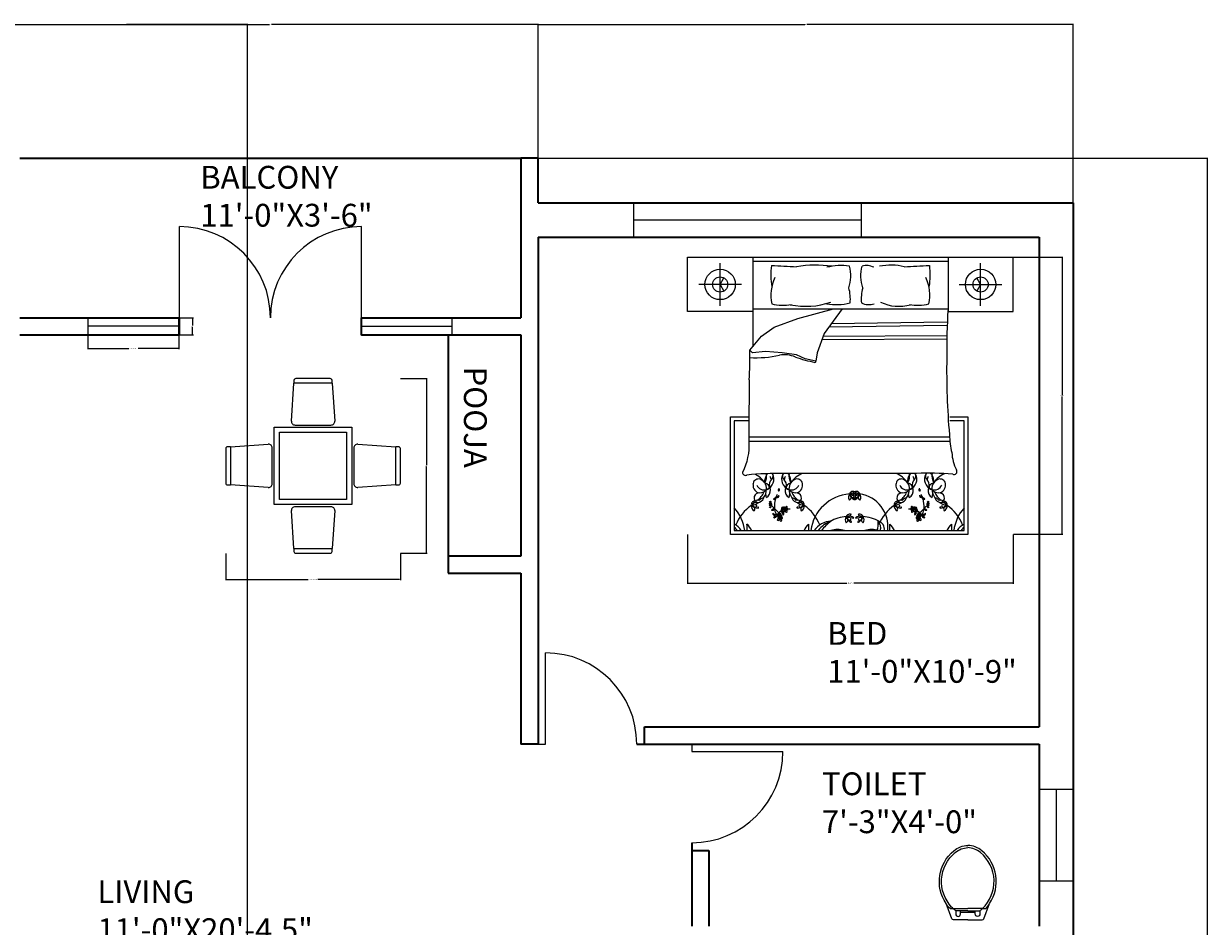
# Model space of a CAD drawing. Units: inches. Extents: x -59 to 444, y -680 to 63.
# Tile 9 of 9: x 132 to 444, y -175 to 63. Entities that reach past the tile are written whole.
import ezdxf

# ---------------------------------------------------------------- set-up
doc = ezdxf.new("R2010")
doc.units = ezdxf.units.IN
doc.header["$MEASUREMENT"] = 0
for name, color, linetype, lineweight in [('A-ANNO-DIMS', 2, 'Continuous', 18), ('A-AREA-IDEN', 7, 'Continuous', 18), ('A-DOOR', 3, 'Continuous', 18), ('A-FLOR-FIXT', 9, 'Continuous', 18), ('A-FURN', 8, 'Continuous', 13), ('A-GLAZ', 4, 'Continuous', 18), ('A-WALL', 7, 'Continuous', 35)]:
    doc.layers.add(name, color=color, linetype=linetype, lineweight=lineweight)
doc.styles.get("Standard").update_dxf_attribs({"font": 'arial.ttf'})
doc.dimstyles.get("Standard").update_dxf_attribs({"dimtxt": 0.18, "dimasz": 0.18, "dimexe": 0.18, "dimexo": 0.0625, "dimgap": 0.09, "dimtad": 0, "dimtih": 1, "dimtoh": 1, "dimdec": 0, "dimzin": 0, "dimdsep": 46, "dimlunit": 3, "dimtxsty": 'Standard', "dimcen": 0.09, "dimadec": 0, "dimazin": 0, "dimtfac": 1, "dimtdec": 0, "dimtofl": 0, "dimtmove": 0, "dimatfit": 3, "dimfxl": 1, "dimtolj": 1, "dimtzin": 0, "dimarcsym": 0})

# ---------------------------------------------------------------- blocks, each defined once
blk = doc.blocks.new('BED-SET-73')
for p, q in [((0, 72.95), (85.77, 72.95)), ((17.15, 72.95), (17.15, 49.4)), ((68.62, 71.84), (17.15, 71.84)), ((8.58, 60.19), (8.58, 71.4)), ((77.2, 60.19), (77.2, 71.4)), ((14.18, 65.8), (2.97, 65.8)), ((71.59, 65.8), (82.8, 65.8)), ((17.15, 59.39), (68.62, 59.39)), ((29.07, 56.84), (38.42, 59.39)), ((40.72, 59.39), (36.02, 52.85)), ((22.81, 54.58), (29.07, 56.84)), ((19.51, 52.15), (22.81, 54.58)), ((68.36, 54.95), (37.21, 54.51)), ((68.39, 55.83), (37.85, 55.4)), ((16.39, 48.51), (19.51, 52.15)), ((36.02, 52.85), (34.11, 47.81)), ((68.32, 51.37), (35.4, 51.23)), ((68.31, 52.25), (35.74, 52.12)), ((17.08, 47.81), (16.39, 48.51)), ((20.56, 48.16), (17.08, 47.81)), ((24.9, 47.81), (20.56, 48.16)), ((28.72, 47.29), (24.9, 47.81)), ((30.98, 46.25), (28.72, 47.29)), ((34.11, 47.81), (33.76, 45.56)), ((33.76, 45.56), (30.98, 46.25)), ((11.32, 30.9), (16.17, 30.9)), ((11.32, 0), (11.32, 30.9)), ((16.17, 29.9), (12.32, 29.9)), ((12.32, 29.9), (12.32, 0.99)), ((72.86, 29.9), (69.08, 29.9)), ((69.1, 30.9), (73.85, 30.9)), ((72.86, 0.99), (72.86, 29.9)), ((73.85, 30.9), (73.85, 0)), ((69.01, 25.55), (16.17, 25.55)), ((69.09, 24.48), (16.17, 24.48)), ((60.3, 16.05), (25.47, 16.05)), ((20.77, 9.69), (20.58, 10.66)), ((26.76, 9.69), (26.95, 10.66)), ((58.41, 9.69), (58.22, 10.66)), ((64.41, 9.69), (64.6, 10.66)), ((73.85, 0), (11.32, 0)), ((12.32, 0.99), (72.86, 0.99))]:
    blk.add_line(p, q)
for points in [[(17.15, 58.65), (0, 58.65), (0, 72.95)], [(68.62, 72.95), (68.62, 58.65), (85.77, 58.65), (85.77, 72.95)], [(8.58, 65.8), (9.58, 67.53)], [(8.58, 65.8), (9.58, 64.06)], [(77.2, 65.8), (76.2, 67.53)], [(77.2, 65.8), (76.2, 64.06)]]:
    blk.add_lwpolyline(points)
for points in [[(22.08, 70.81, 0.074897), (22.19, 65.21, -0.472817)], [(42.49, 64.89, 0.14099), (42.66, 70.61, 0.235245)], [(46.15, 64.89, -0.14099), (45.98, 70.61, -0.235245)], [(63.69, 70.81, -0.074897), (63.59, 65.21, 0.472817)], [(16.21, 40.65, 0.001242), (16.17, 24.38, -0.127202), (14.45, 16.27)], [(68.99, 26.22, 0.056112), (69.61, 21.51, 0.095341), (70.81, 16.96)]]:
    blk.add_lwpolyline(points, format="xyb")
for centre, radius in [((8.58, 65.8), 4), ((77.2, 65.8), 4), ((8.58, 65.8), 2), ((77.2, 65.8), 2), ((25.72, 6.58), 0.218), ((59.45, 6.58), 0.218), ((24.29, 4.28), 0.218), ((60.88, 4.28), 0.218)]:
    blk.add_circle(centre, radius)
for centre, radius, start, end in [((69.36, 887.1), 817.66, 266.68521, 267.14978), ((33.83, 39.77), 31.11, 82.2196, 99.497), ((40.4, 55.49), 15.28, 81.5249, 103.96), ((47.15, 66.53), 4.24, 63.3437, 106.1026), ((53.51, 55.8), 15.08, 76.3427, 101.1841), ((16.41, 887.1), 817.66, 272.85022, 273.31479), ((33.01, 62.96), 11.06, 155.1316, 191.7583), ((52.76, 62.96), 11.06, 348.2417, 24.8684), ((32.37, 62.02), 10.51, 354.0129, 15.8293), ((56.26, 62.02), 10.51, 164.1707, 185.9871), ((25.14, 71.81), 11.49, 255.1039, 281.0369), ((31.19, 79.98), 19.94, 258.0397, 289.2615), ((39.26, 75.63), 15.13, 259.8617, 283.6238), ((47.73, 65.05), 4.55, 245.0183, 288.5407), ((55.67, 70.96), 10.92, 243.8761, 286.1746), ((60.63, 71.81), 11.49, 258.9631, 284.8961), ((222.38, 48.91), 154.12, 176.1, 180.9282), ((-62.26, 46.38), 78.68, 355.8294, 1.553), ((17.85, 78.88), 32.37, 267.4519, 281.3392), ((25.59, 40.3), 6.98, 66.2616, 101.3392), ((39.72, 77.97), 33.26, 250.1194, 259.3383), ((33.57, 45.49), 0.207, 268.8623, 19.7536), ((269.3, 43.3), 201.05, 179.1145, 184.8735), ((15.24, 16.32), 0.791, 183.98, 297.3412), ((24.45, -73.23), 89.29, 89.3433, 95.6887), ((14.9, 10.01), 6.49, 33.6671, 63.2997), ((23.6, 13.88), 3.31, 145.785, 184.7304), ((17.28, 15.42), 3.55, 328.8218, 9.1554), ((21.68, 15.1), 1.03, 120.0293, 142.325), ((20.04, 14.5), 2.73, 289.2822, 29.1751), ((21.25, 15.31), 1.28, 311.5653, 23.8354), ((21.68, 15.1), 1.03, 44.4517, 63.558), ((27.5, 14.5), 2.73, 150.8249, 250.7178), ((26.28, 15.31), 1.28, 156.1646, 228.4347), ((25.85, 15.1), 1.03, 113.229, 135.5483), ((25.85, 15.1), 1.03, 37.675, 66.7144), ((23.93, 13.88), 3.31, 355.2696, 34.215), ((30.25, 15.42), 3.55, 169.7133, 211.1782), ((32.63, 10.01), 6.49, 111.4941, 146.3329), ((52.55, 10.01), 6.49, 33.6671, 68.5059), ((61.25, 13.88), 3.31, 145.785, 184.7304), ((54.93, 15.42), 3.55, 328.8218, 10.2867), ((59.33, 15.1), 1.03, 113.2856, 142.325), ((57.68, 14.5), 2.73, 289.2822, 29.1751), ((59.33, 15.1), 1.03, 44.4517, 66.7144), ((58.89, 15.31), 1.28, 311.5653, 23.8354), ((62.93, -67.37), 83.47, 85.2402, 91.8035), ((65.14, 14.5), 2.73, 150.8249, 250.7178), ((63.93, 15.31), 1.28, 156.1646, 228.4347), ((63.49, 15.1), 1.03, 106.6343, 135.5483), ((63.49, 15.1), 1.03, 37.675, 72.5814), ((61.57, 13.88), 3.31, 355.2696, 34.215), ((67.89, 15.42), 3.55, 169.249, 211.1782), ((70.27, 10.01), 6.49, 113.6453, 146.3329), ((70.16, 16.52), 0.782, 246.5219, 33.8264), ((19.28, 12.92), 2.05, 174.9449, 262.8857), ((18.68, 13.13), 1.45, 84.4856, 181.0538), ((20.08, 13.7), 1.99, 201.5819, 291.4221), ((18.24, 12.06), 2.58, 355.2933, 76.921), ((19.7, 11.54), 2.13, 299.9085, 73.1337), ((21.05, 12.43), 0.532, 257.3041, 15.1471), ((23.27, 13.03), 1.76, 131.5653, 195.1471), ((19.62, 14), 2.47, 7.436, 29.9149), ((24.26, 13.03), 1.76, 344.8529, 48.4347), ((27.91, 14), 2.47, 150.0851, 172.564), ((27.83, 11.54), 2.13, 106.8663, 240.0915), ((26.48, 12.43), 0.532, 164.8529, 282.6959), ((29.29, 12.06), 2.58, 103.079, 184.7067), ((27.45, 13.7), 1.99, 248.5779, 338.4181), ((28.25, 12.92), 2.05, 277.1143, 5.0551), ((28.85, 13.13), 1.45, 358.9462, 95.5144), ((56.92, 12.92), 2.05, 174.9449, 262.8857), ((56.33, 13.13), 1.45, 84.4856, 181.0538), ((57.73, 13.7), 1.99, 201.5819, 291.4221), ((55.88, 12.06), 2.58, 355.2933, 76.921), ((57.35, 11.54), 2.13, 299.9085, 73.1337), ((58.7, 12.43), 0.532, 257.3041, 15.1471), ((60.91, 13.03), 1.76, 131.5653, 195.1471), ((57.27, 14), 2.47, 7.436, 29.9149), ((61.91, 13.03), 1.76, 344.8529, 48.4347), ((65.55, 14), 2.47, 150.0851, 172.564), ((65.47, 11.54), 2.13, 106.8663, 240.0915), ((64.12, 12.43), 0.532, 164.8529, 282.6959), ((66.94, 12.06), 2.58, 103.079, 184.7067), ((65.09, 13.7), 1.99, 248.5779, 338.4181), ((65.9, 12.92), 2.05, 277.1143, 5.0551), ((66.49, 13.13), 1.45, 358.9462, 95.5144), ((18.81, 9.62), 1.29, 80.264, 250.8688), ((16.25, 12.45), 4.05, 301.2614, 341.7045), ((18.5, 10.01), 1.61, 265.969, 344.3045), ((20.23, 7.87), 1.71, 96.1662, 141.5825), ((18.92, 13.38), 2.49, 272.3591, 324.0401), ((16.22, 12.13), 4.6, 326.2883, 356.5076), ((23.6, 13.88), 3.31, 212.7011, 216.3445), ((23.06, 9.07), 0.45, 101.3256, 154.4621), ((22.42, 10.6), 1.36, 280.2588, 300.656), ((22.12, 10.6), 1.38, 308.2101, 316.3071), ((22.97, 9.69), 0.412, 278.3432, 4.2869), ((22.74, 10.05), 0.719, 300.656, 332.6341), ((23.28, 9.58), 0.175, 55.7657, 157.4417), ((29.96, 7.31), 7.1, 153.0032, 159.8941), ((23.55, 9.74), 0.175, 84.3784, 186.0543), ((23.39, 10.44), 0.719, 269.1859, 301.164), ((23.6, 10.07), 0.412, 237.5332, 323.4768), ((23.2, 11.24), 1.38, 285.5129, 293.6099), ((24.1, 9.69), 0.45, 87.3579, 140.4944), ((23.06, 10.99), 1.36, 301.164, 321.5612), ((24.01, 11.63), 0.165, 102.7051, 280.4384), ((21.96, 11.22), 2.42, 324.6898, 333.4936), ((23.99, 11.73), 0.269, 280.4384, 100.4136), ((23.93, 13.88), 3.31, 323.6555, 327.2989), ((28.61, 13.38), 2.49, 215.9599, 267.6409), ((31.31, 12.13), 4.6, 183.4924, 213.7117), ((31.28, 12.45), 4.05, 198.2955, 238.7386), ((27.3, 7.87), 1.71, 38.4175, 83.8338), ((29.03, 10.01), 1.61, 195.6955, 274.031), ((28.72, 9.62), 1.29, 289.1312, 99.736), ((43.55, -0.52), 11.2, 94.4623, 172.255), ((43.6, 9.82), 1.24, 137.7873, 219.1145), ((42.19, 9.86), 0.935, 298.5391, 58.3627), ((43.57, 10.39), 0.929, 63.0274, 163.8037), ((42.63, 12.56), 1.91, 271.4585, 315.3727), ((43.41, 9.04), 1.77, 45.5411, 114.3101), ((45.03, 18.13), 7.84, 252.593, 267.2582), ((43.6, 10.62), 0.916, 177.7585, 283.852), ((45.36, 11.57), 2.83, 198.9159, 238.011), ((44.62, 9.04), 1.77, 65.6899, 134.4589), ((43.01, 18.13), 7.84, 272.7418, 287.407), ((43.79, 9.84), 0.121, 283.852, 219.9245), ((43.94, 9.29), 0.139, 238.011, 71.5592), ((43.96, 9.35), 0.0676, 71.5592, 188.0167), ((44.1, 9.29), 0.139, 108.4408, 301.989), ((44.46, 10.39), 0.929, 16.1963, 116.9726), ((45.4, 12.56), 1.91, 224.6273, 268.5415), ((44.08, 9.35), 0.0676, 351.9833, 108.4408), ((44.23, 9.89), 0.073, 320.1909, 256.0209), ((42.67, 11.57), 2.83, 301.989, 341.0841), ((44.44, 10.62), 0.916, 256.148, 2.2415), ((45.84, 9.86), 0.935, 121.6373, 241.4609), ((44.43, 9.82), 1.24, 320.8855, 42.2127), ((44.12, 2.07), 8.67, 352.8636, 81.8197), ((56.45, 9.62), 1.29, 80.264, 250.8688), ((53.9, 12.45), 4.05, 301.2614, 341.7045), ((56.14, 10.01), 1.61, 265.969, 344.3045), ((57.87, 7.87), 1.71, 96.1662, 141.5825), ((56.57, 13.38), 2.49, 272.3591, 324.0401), ((53.86, 12.13), 4.6, 326.2883, 356.5076), ((61.25, 13.88), 3.31, 212.7011, 216.3445), ((61.18, 11.73), 0.269, 79.5864, 259.5616), ((62.12, 10.99), 1.36, 218.4388, 238.836), ((61.07, 9.69), 0.45, 39.5056, 92.6421), ((63.22, 11.22), 2.42, 206.5064, 215.3102), ((61.16, 11.63), 0.165, 259.5616, 77.2949), ((61.58, 10.07), 0.412, 216.5232, 302.4668), ((61.79, 10.44), 0.719, 238.836, 270.8141), ((61.97, 11.24), 1.38, 246.3901, 254.4871), ((55.22, 7.31), 7.1, 20.1059, 26.9968), ((61.62, 9.74), 0.175, 353.9457, 95.6216), ((61.89, 9.58), 0.175, 22.5583, 124.2343), ((62.21, 9.69), 0.412, 175.7131, 261.6568), ((62.43, 10.05), 0.719, 207.3659, 239.344), ((63.05, 10.6), 1.38, 223.6929, 231.7899), ((62.76, 10.6), 1.36, 239.344, 259.7412), ((62.11, 9.07), 0.45, 25.5379, 78.6744), ((61.57, 13.88), 3.31, 323.6555, 327.2989), ((66.25, 13.38), 2.49, 215.9599, 267.6409), ((68.96, 12.13), 4.6, 183.4924, 213.7117), ((68.92, 12.45), 4.05, 198.2955, 238.7386), ((66.68, 10.01), 1.61, 195.6955, 274.031), ((64.95, 7.87), 1.71, 38.4175, 83.8338), ((66.37, 9.62), 1.29, 289.1312, 99.736), ((3.98, -0.52), 11.2, 7.745, 41.8856), ((23.14, -1.62), 11.2, 124.3865, 158.5908), ((18.03, 7.36), 1.24, 167.7115, 249.0387), ((17.72, 7.84), 0.929, 92.9516, 193.728), ((15.82, 9.25), 1.91, 301.3827, 345.2969), ((18.25, 6.59), 1.77, 75.4653, 144.2343), ((15.12, 15.27), 7.84, 282.5173, 297.1824), ((16.79, 6.69), 0.935, 328.4633, 88.2869), ((18.68, 9.75), 2.83, 228.8402, 267.9352), ((17.62, 8.05), 0.916, 207.6827, 313.7762), ((18.54, 8.23), 0.789, 63.9755, 143.2681), ((18.17, 7.47), 0.121, 313.7762, 249.7183), ((18.57, 7.13), 0.0676, 101.4834, 217.9409), ((18.58, 7.06), 0.139, 267.9352, 101.4834), ((21.79, 8.22), 0.364, 101.5637, 142.6358), ((21.49, 7.88), 0.218, 273.2768, 86.7232), ((21.79, 7.48), 0.361, 217.7621, 259.0403), ((21.74, 8.09), 0.209, 91.1081, 181.8675), ((22.18, 7.96), 0.663, 203.4276, 227.6104), ((21.96, 7.67), 0.452, 80.3487, 133.6538), ((21.88, 8.04), 0.357, 229.7889, 317.6792), ((21.5, 8.5), 0.525, 288.7263, 352.5032), ((21.48, 7.28), 0.508, 355.053, 68.3618), ((21.88, 7.2), 0.715, 83.0852, 105.7171), ((21.86, 8.48), 0.169, 345.2356, 144.9248), ((21.82, 7.25), 0.168, 232.4737, 355.053), ((16.93, 1.27), 8.14, 43.1541, 52.0459), ((22.01, 7.93), 0.188, 317.6792, 80.3487), ((22.55, 6.19), 0.45, 101.3256, 154.4621), ((21.91, 7.71), 1.36, 280.2588, 300.656), ((22.22, 8.8), 2.42, 268.3264, 277.1302), ((21.61, 7.71), 1.38, 308.2101, 316.3071), ((22.46, 6.81), 0.412, 278.3432, 4.2869), ((22.23, 7.17), 0.719, 300.656, 332.6341), ((22.77, 6.69), 0.175, 55.7657, 157.4417), ((22.73, 11.68), 2.42, 268.3264, 277.1302), ((29.96, 7.31), 7.1, 163.5842, 183.8277), ((26.42, 7.13), 3.56, 184.756, 209.2041), ((31.54, 14.71), 11.72, 222.2412, 232.1744), ((24.58, 6.68), 0.605, 272.8499, 356.1226), ((24.05, 6.91), 0.996, 304.5369, 16.3699), ((24.16, 6.45), 0.586, 321.7607, 7.9252), ((25.43, 6.63), 0.704, 127.3105, 187.9252), ((24.47, 6.71), 0.723, 355.0106, 41.658), ((25.26, 6.17), 0.216, 148.0499, 225.6268), ((26.78, 2.4), 4.27, 113.0501, 113.8477), ((25.66, 5.92), 0.689, 104.7558, 148.0499), ((25.28, 6.42), 0.431, 247.4086, 351.4386), ((25.48, 6.89), 0.298, 126.1046, 271.4281), ((25.45, 6.97), 0.214, 353.7526, 131.7054), ((25.4, 6.4), 0.145, 262.906, 7.132), ((25.25, 6.71), 0.301, 0.0645, 61.1507), ((25.32, 6.97), 0.344, 311.8413, 355.7877), ((26.03, 6.92), 0.364, 101.5637, 176.365), ((26.02, 6.18), 0.361, 151.2196, 259.0403), ((25.98, 6.79), 0.209, 91.1081, 181.8675), ((26.41, 6.66), 0.663, 203.4276, 227.6104), ((26.2, 6.37), 0.452, 80.3487, 133.6538), ((26.12, 6.74), 0.357, 229.7889, 317.6792), ((25.73, 7.21), 0.525, 288.7263, 352.5032), ((25.72, 5.99), 0.508, 355.053, 68.3618), ((26.11, 5.9), 0.715, 83.0852, 105.7171), ((26.09, 7.18), 0.169, 345.2356, 144.9248), ((26.24, 6.63), 0.188, 317.6792, 80.3487), ((26.78, 2.4), 4.27, 87.1071, 94.7585), ((28.99, 8.23), 0.789, 36.7319, 116.0245), ((28.95, 7.06), 0.139, 78.5166, 272.0648), ((29.28, 6.59), 1.77, 35.7657, 104.5347), ((32.42, 15.27), 7.84, 242.8176, 257.4827), ((28.85, 9.75), 2.83, 272.0648, 311.1598), ((28.96, 7.13), 0.0676, 322.0591, 78.5166), ((29.91, 8.05), 0.916, 226.2238, 332.3173), ((29.37, 7.52), 0.073, 290.2667, 226.2271), ((30.74, 6.69), 0.935, 91.7131, 211.5367), ((29.81, 7.84), 0.929, 346.272, 87.0484), ((31.71, 9.25), 1.91, 194.7031, 238.6173), ((29.5, 7.36), 1.24, 290.9613, 12.2885), ((24.39, -1.62), 11.2, 21.4092, 55.6135), ((60.78, -1.62), 11.2, 124.3865, 158.5908), ((55.36, 7.84), 0.929, 92.9516, 193.728), ((55.67, 7.36), 1.24, 167.7115, 249.0387), ((53.46, 9.25), 1.91, 301.3827, 345.2969), ((55.9, 6.59), 1.77, 75.4653, 144.2343), ((52.76, 15.27), 7.84, 282.5173, 297.1824), ((55.27, 8.05), 0.916, 207.6827, 313.7762), ((56.32, 9.75), 2.83, 228.8402, 267.9352), ((54.43, 6.69), 0.935, 328.4633, 88.2869), ((56.19, 8.23), 0.789, 63.9755, 143.2681), ((55.82, 7.47), 0.121, 313.7762, 249.7183), ((56.21, 7.13), 0.0676, 101.4834, 217.9409), ((56.23, 7.06), 0.139, 267.9352, 101.4834), ((58.39, 2.4), 4.27, 85.2415, 92.8929), ((58.93, 6.63), 0.188, 99.6513, 222.3208), ((59.06, 6.74), 0.357, 222.3208, 310.2111), ((58.98, 6.37), 0.452, 46.3462, 99.6513), ((59.09, 7.18), 0.169, 35.0752, 194.7644), ((59.44, 7.21), 0.525, 187.4968, 251.2737), ((59.46, 5.99), 0.508, 111.6382, 184.947), ((59.06, 5.9), 0.715, 74.2829, 96.9148), ((59.2, 6.79), 0.209, 358.1325, 88.8919), ((58.77, 6.66), 0.663, 312.3896, 336.5724), ((59.15, 6.92), 0.364, 3.635, 78.4363), ((59.15, 6.18), 0.361, 280.9597, 28.7804), ((59.9, 6.42), 0.431, 188.5614, 292.5914), ((59.73, 6.97), 0.214, 48.2946, 186.2474), ((59.86, 6.97), 0.344, 184.2123, 228.1587), ((59.93, 6.71), 0.301, 118.8493, 179.9355), ((59.78, 6.4), 0.145, 172.868, 277.094), ((59.69, 6.89), 0.298, 268.5719, 53.8954), ((59.51, 5.92), 0.689, 31.9501, 75.2442), ((60.71, 6.71), 0.723, 138.342, 184.9894), ((60.59, 6.68), 0.605, 183.8774, 267.1501), ((58.39, 2.4), 4.27, 66.1523, 66.9499), ((59.91, 6.17), 0.216, 314.3732, 31.9501), ((61.12, 6.91), 0.996, 163.6301, 235.4631), ((59.74, 6.63), 0.704, 352.0748, 52.6895), ((61.02, 6.45), 0.586, 172.0748, 218.2393), ((53.63, 14.71), 11.72, 307.8256, 317.7588), ((58.76, 7.13), 3.56, 330.7959, 355.244), ((55.22, 7.31), 7.1, 356.1723, 16.4158), ((62.45, 11.68), 2.42, 262.8698, 271.6736), ((68.25, 1.27), 8.14, 127.9541, 136.8459), ((62.41, 6.69), 0.175, 22.5583, 124.2343), ((62.72, 6.81), 0.412, 175.7131, 261.6568), ((62.95, 7.17), 0.719, 207.3659, 239.344), ((63.56, 7.71), 1.38, 223.6929, 231.7899), ((63.27, 7.71), 1.36, 239.344, 259.7412), ((62.96, 8.8), 2.42, 262.8698, 271.6736), ((62.62, 6.19), 0.45, 25.5379, 78.6744), ((63.17, 7.93), 0.188, 99.6513, 222.3208), ((63.29, 8.04), 0.357, 222.3208, 310.2111), ((63.21, 7.67), 0.452, 46.3462, 99.6513), ((63.32, 8.48), 0.169, 35.0752, 194.7644), ((63.68, 8.5), 0.525, 187.4968, 251.2737), ((63.69, 7.28), 0.508, 111.6382, 184.947), ((63.36, 7.25), 0.168, 184.947, 307.5263), ((63.3, 7.2), 0.715, 74.2829, 96.9148), ((63.43, 8.09), 0.209, 358.1325, 88.8919), ((63, 7.96), 0.663, 312.3896, 336.5724), ((63.38, 8.22), 0.364, 37.3642, 78.4363), ((63.39, 7.48), 0.361, 280.9597, 322.2379), ((63.69, 7.88), 0.218, 93.2768, 266.7232), ((66.63, 8.23), 0.789, 36.7319, 116.0245), ((66.59, 7.06), 0.139, 78.5166, 272.0648), ((66.93, 6.59), 1.77, 35.7657, 104.5347), ((70.06, 15.27), 7.84, 242.8176, 257.4827), ((66.5, 9.75), 2.83, 272.0648, 311.1598), ((66.61, 7.13), 0.0676, 322.0591, 78.5166), ((67.55, 8.05), 0.916, 226.2238, 332.3173), ((67.01, 7.52), 0.073, 290.2667, 226.2271), ((68.39, 6.69), 0.935, 91.7131, 211.5367), ((69.36, 9.25), 1.91, 194.7031, 238.6173), ((67.46, 7.84), 0.929, 346.272, 87.0484), ((67.15, 7.36), 1.24, 290.9613, 12.2885), ((62.04, -1.62), 11.2, 21.4092, 55.6135), ((81.2, -0.52), 11.2, 138.1144, 172.255), ((22.71, 5.4), 0.244, 146.8636, 236.9021), ((26.14, 10.77), 6.38, 235.1882, 238.8844), ((23.12, 5.75), 0.66, 199.4799, 267.6828), ((23.05, 5.5), 0.569, 212.8155, 277.3992), ((22.72, 5.12), 0.66, 266.9701, 338.2913), ((19.24, 9.83), 6.38, 302.6784, 306.3746), ((22.89, 4.6), 0.244, 214.3538, 304.3923), ((22.98, 5.52), 0.253, 238.8844, 314.2646), ((22.92, 4.96), 0.569, 280.3057, 17.1958), ((22.87, 4.9), 0.253, 306.3746, 21.7548), ((23.29, 5.06), 0.191, 19.3605, 201.7548), ((23.29, 5.2), 0.191, 311.8703, 134.2646), ((26.87, 3.47), 3.8, 153.7819, 158.2913), ((23.84, 6.07), 0.996, 247.2305, 319.0635), ((23.51, 5.73), 0.586, 264.4544, 310.6188), ((23.94, 5.5), 0.605, 218.3208, 298.8162), ((26.42, 7.13), 3.56, 214.0033, 222.4917), ((26.78, 2.4), 4.27, 120.544, 139.818), ((23.84, 3.87), 0.216, 148.0499, 225.6268), ((24.24, 3.62), 0.689, 104.7558, 148.0499), ((23.85, 4.11), 0.431, 247.4086, 351.4386), ((24.05, 4.58), 0.298, 126.1046, 271.4281), ((24.02, 4.66), 0.214, 353.7526, 131.7054), ((24.35, 4.75), 0.704, 70.0041, 130.6188), ((23.97, 4.1), 0.145, 262.906, 7.132), ((23.82, 4.41), 0.301, 0.0645, 61.1507), ((23.89, 4.67), 0.344, 311.8413, 355.7877), ((23.89, 5.61), 0.723, 297.7043, 344.3516), ((24.6, 4.62), 0.364, 101.5637, 176.365), ((24.59, 3.88), 0.361, 151.2196, 259.0403), ((24.55, 4.49), 0.209, 91.1081, 181.8675), ((24.98, 4.36), 0.663, 203.4276, 227.6104), ((24.77, 4.07), 0.452, 80.3487, 133.6538), ((24.69, 4.44), 0.357, 229.7889, 317.6792), ((24.3, 4.9), 0.525, 288.7263, 352.5032), ((24.29, 3.68), 0.508, 355.053, 68.3618), ((24.68, 3.6), 0.715, 83.0852, 105.7171), ((24.66, 4.88), 0.169, 345.2356, 144.9248), ((24.63, 3.65), 0.168, 232.4737, 355.053), ((24.28, 5.61), 0.586, 8.7227, 54.8872), ((24.31, 5.14), 0.996, 0.278, 72.111), ((24.76, 5.5), 0.605, 20.5253, 88.5375), ((24.81, 4.33), 0.188, 317.6792, 80.3487), ((25.55, 5.8), 0.704, 188.7227, 249.3375), ((24.65, 5.45), 0.723, 334.9899, 21.6373), ((26.05, 5.96), 0.168, 232.4737, 355.053), ((37.93, -2.02), 5.46, 91.272, 146.5383), ((39.9, -3.03), 6.8, 107.8504, 143.6964), ((43.47, -4.95), 10.12, 124.0123, 144.053), ((42.7, -6.51), 11.2, 94.4623, 117.4146), ((42.74, 3.82), 1.24, 137.7873, 219.1145), ((41.33, 3.86), 0.935, 298.5391, 58.3627), ((42.72, 4.39), 0.929, 63.0274, 163.8037), ((41.78, 6.56), 1.91, 271.4585, 315.3727), ((42.55, 3.04), 1.77, 45.5411, 114.3101), ((44.5, 5.57), 2.83, 198.9159, 238.011), ((44.17, 12.13), 7.84, 252.593, 267.2582), ((42.74, 4.62), 0.916, 177.7585, 283.852), ((42.93, 3.84), 0.121, 283.852, 219.9245), ((43.08, 3.29), 0.139, 238.011, 71.5592), ((43.1, 3.35), 0.0676, 71.5592, 188.0167), ((45.48, 3.04), 1.77, 65.6899, 134.4589), ((43.87, 12.13), 7.84, 272.7418, 287.407), ((44.96, 3.29), 0.139, 108.4408, 301.989), ((45.32, 4.39), 0.929, 16.1963, 116.9726), ((46.26, 6.56), 1.91, 224.6273, 268.5415), ((44.93, 3.35), 0.0676, 351.9833, 108.4408), ((45.09, 3.89), 0.073, 320.1909, 256.0209), ((43.53, 5.57), 2.83, 301.989, 341.0841), ((45.29, 4.62), 0.916, 256.148, 2.2415), ((46.7, 3.86), 0.935, 121.6373, 241.4609), ((45.29, 3.82), 1.24, 320.8855, 42.2127), ((45.34, -6.51), 11.2, 62.5854, 85.5377), ((45.24, 2.86), 5.01, 338.117, 6.6195), ((49.84, 1.47), 2.01, 346.3898, 79.0739), ((48.33, 1.74), 2.54, 342.8609, 41.9049), ((59.12, 5.96), 0.168, 184.947, 307.5263), ((60.53, 5.45), 0.723, 158.3627, 205.0101), ((60.42, 5.5), 0.605, 91.4625, 159.4747), ((60.87, 5.14), 0.996, 107.889, 179.722), ((59.62, 5.8), 0.704, 290.6625, 351.2773), ((60.36, 4.33), 0.188, 99.6513, 222.3208), ((60.49, 4.44), 0.357, 222.3208, 310.2111), ((60.9, 5.61), 0.586, 125.1128, 171.2773), ((60.4, 4.07), 0.452, 46.3462, 99.6513), ((60.51, 4.88), 0.169, 35.0752, 194.7644), ((60.87, 4.9), 0.525, 187.4968, 251.2737), ((60.89, 3.68), 0.508, 111.6382, 184.947), ((60.55, 3.65), 0.168, 184.947, 307.5263), ((60.49, 3.6), 0.715, 74.2829, 96.9148), ((58.39, 2.4), 4.27, 40.182, 59.456), ((60.82, 4.75), 0.704, 49.3812, 109.9959), ((61.34, 6.07), 0.996, 220.9365, 292.7695), ((61.28, 5.61), 0.723, 195.6484, 242.2957), ((60.63, 4.49), 0.209, 358.1325, 88.8919), ((60.19, 4.36), 0.663, 312.3896, 336.5724), ((60.58, 4.62), 0.364, 3.635, 78.4363), ((60.58, 3.88), 0.361, 280.9597, 28.7804), ((61.33, 4.11), 0.431, 188.5614, 292.5914), ((61.24, 5.5), 0.605, 241.1838, 321.6792), ((61.16, 4.66), 0.214, 48.2946, 186.2474), ((61.29, 4.67), 0.344, 184.2123, 228.1587), ((61.36, 4.41), 0.301, 118.8493, 179.9355), ((61.2, 4.1), 0.145, 172.868, 277.094), ((61.12, 4.58), 0.298, 268.5719, 53.8954), ((60.94, 3.62), 0.689, 31.9501, 75.2442), ((61.66, 5.73), 0.586, 229.3812, 275.5456), ((58.76, 7.13), 3.56, 317.5083, 325.9967), ((61.34, 3.87), 0.216, 314.3732, 31.9501), ((62.25, 4.96), 0.569, 162.8042, 259.6943), ((61.89, 5.2), 0.191, 45.7354, 228.1297), ((61.89, 5.06), 0.191, 338.2452, 160.6395), ((58.31, 3.47), 3.8, 21.7087, 26.2181), ((62.46, 5.12), 0.66, 201.7087, 273.0299), ((62.2, 5.52), 0.253, 225.7354, 301.1156), ((62.13, 5.5), 0.569, 262.6008, 327.1845), ((62.3, 4.9), 0.253, 158.2452, 233.6254), ((62.05, 5.75), 0.66, 272.3172, 340.5201), ((65.94, 9.83), 6.38, 233.6254, 237.3216), ((62.29, 4.6), 0.244, 235.6077, 325.6462), ((59.03, 10.77), 6.38, 301.1156, 304.8118), ((62.47, 5.4), 0.244, 303.0979, 33.1364), ((9.6, -2.02), 5.46, 33.4617, 60.1116), ((7.63, -3.03), 6.8, 36.3036, 46.4814), ((12.65, -0.75), 4.55, 22.5547, 48.9546), ((0.18, 1.69), 15.5, 357.4081, 3.6519), ((34.88, -0.75), 4.55, 131.0454, 157.4453), ((47.35, 1.69), 15.5, 176.3481, 182.5919), ((39.56, -4.9), 6.16, 73.5431, 107.0202), ((42, -8.07), 9.11, 94.3787, 95.6357), ((46.8, -14.31), 16.28, 109.7217, 109.9028), ((48.47, -4.9), 6.16, 72.9798, 106.4569), ((46.03, -8.07), 9.11, 84.3643, 85.6213), ((41.23, -14.31), 16.28, 70.0972, 70.2783), ((37.82, 1.69), 15.5, 357.4081, 3.6519), ((50.3, -0.75), 4.55, 22.5547, 48.9546), ((72.52, -0.75), 4.55, 131.0454, 157.4453), ((85, 1.69), 15.5, 176.3481, 182.5919), ((75.58, -2.02), 5.46, 119.8884, 146.5383), ((77.54, -3.03), 6.8, 133.5186, 143.6964)]:
    blk.add_arc(centre, radius, start, end)
blk = doc.blocks.new('DINING-SET-4')
for p, q in [((17.3, 34.79), (17.98, 44.78)), ((17.98, 45.52), (17.98, 44.78)), ((28.03, 44.78), (17.98, 44.78)), ((27.54, 46.01), (18.47, 46.01)), ((28.03, 44.78), (28.03, 45.52)), ((28.03, 44.78), (28.7, 34.79)), ((18.28, 33.76), (27.73, 33.76)), ((1.22, 28.03), (11.22, 28.71)), ((34.79, 28.71), (44.78, 28.03)), ((0, 27.54), (0, 18.47)), ((1.22, 28.03), (0.49, 28.03)), ((1.22, 28.03), (1.22, 17.98)), ((12.25, 18.28), (12.25, 27.73)), ((33.76, 27.73), (33.76, 18.28)), ((45.52, 28.03), (44.78, 28.03)), ((44.78, 17.98), (44.78, 28.03)), ((46.01, 18.47), (46.01, 27.54)), ((0.49, 17.98), (1.22, 17.98)), ((11.22, 17.3), (1.22, 17.98)), ((44.78, 17.98), (34.79, 17.3)), ((44.78, 17.98), (45.52, 17.98)), ((17.98, 1.23), (17.3, 11.22)), ((27.73, 12.25), (18.28, 12.25)), ((28.7, 11.22), (28.03, 1.23)), ((17.98, 1.23), (28.03, 1.23)), ((17.98, 1.23), (17.98, 0.49)), ((18.47, 0), (27.54, 0)), ((28.03, 0.49), (28.03, 1.23))]:
    blk.add_line(p, q)
for points in [[(12.79, 12.8), (12.79, 33.21), (33.21, 33.21), (33.21, 12.8)], [(14.16, 14.16), (14.16, 31.85), (31.85, 31.85), (31.85, 14.16)]]:
    blk.add_lwpolyline(points, close=True)
for centre, radius, start, end in [((18.47, 45.52), 0.49, 90, 180), ((27.54, 45.52), 0.49, 0, 90), ((18.28, 34.74), 0.98, 176.8779, 270), ((27.73, 34.74), 0.98, 270, 3.1221), ((11.27, 27.73), 0.98, 0, 93.1221), ((34.74, 27.73), 0.98, 86.8779, 180), ((0.49, 27.54), 0.49, 90, 180), ((45.52, 27.54), 0.49, 0, 90), ((0.49, 18.47), 0.49, 180, 270), ((11.27, 18.28), 0.98, 266.8779, 0), ((34.74, 18.28), 0.98, 180, 273.1221), ((45.52, 18.47), 0.49, 270, 0), ((18.28, 11.27), 0.98, 90, 183.1221), ((27.73, 11.27), 0.98, 356.8779, 90), ((18.47, 0.49), 0.49, 180, 270), ((27.54, 0.49), 0.49, 270, 0)]:
    blk.add_arc(centre, radius, start, end)
blk = doc.blocks.new('WC-FLOOR')
for p, q in [((2.81, 2.97), (3.64, 2.97)), ((3.64, 2.97), (7.5, 2.97)), ((11.36, 2.97), (7.5, 2.97)), ((11.36, 2.97), (12.18, 2.97))]:
    blk.add_line(p, q)
for points in [[(1.75, 4.32, -0.383919), (3.81, 18.21, -0.163732), (7.5, 19.62, -0.359733)], [(3.24, 3.37, -0.431639), (4.18, 17.76, -0.162618), (7.5, 19.04, -0.470877)], [(13.24, 4.32, 0.383919), (11.19, 18.21, 0.163732), (7.5, 19.62, 0.359733)], [(11.36, 2.97, 0.448546), (10.81, 17.76, 0.162618), (7.5, 19.04, 0.470877)], [(2.81, 2.97, -0.040937), (1.75, 4.32, -0.163732)], [(7.5, 0), (3.75, 0, -0.31031), (3.29, 0.32), (1.75, 4.32, -0.209071)], [(3.64, 2.97, -0.014165), (3.24, 3.37, -0.162618)], [(7.5, 0), (11.24, 0, 0.31031), (11.7, 0.32), (13.24, 4.32, 0.209071)], [(12.18, 2.97, 0.040937), (13.24, 4.32, 0.163732)], [(4.31, 2.38, -0.022712), (3.64, 2.97, -0.162618)], [(7.5, 2.38), (4.31, 2.38, -0.022712)], [(4.31, 2.38), (4.31, 1.55, 1), (5.56, 1.55), (5.56, 1.98)], [(7.5, 2.38), (10.68, 2.38, 0.476108)], [(10.68, 2.38), (10.68, 1.55, -1), (9.43, 1.55), (9.43, 1.98)], [(10.68, 2.38, 0.022712), (11.36, 2.97, 0.162618)]]:
    blk.add_lwpolyline(points, format="xyb")
for points in [[(5.56, 1.98), (5.56, 2.38)], [(9.43, 1.98), (5.56, 1.98)], [(9.43, 1.98), (9.43, 2.38)]]:
    blk.add_lwpolyline(points)
blk = doc.blocks.new('WIN-60-W9')
for p, q in [((60, 9), (0, 9)), ((0, 9), (0, 0)), ((60, 0), (60, 9)), ((0, 4.5), (60, 4.5)), ((0, 0), (60, 0))]:
    blk.add_line(p, q)
blk = doc.blocks.new('WIN-24-W9')
for p, q in [((0, 24), (0, 0)), ((9, 24), (0, 24)), ((4.5, 24), (4.5, 0)), ((9, 0), (9, 24)), ((0, 0), (9, 0))]:
    blk.add_line(p, q)
blk = doc.blocks.new('WIN-24-W4-5')
for p, q in [((24, 4.5), (0, 4.5)), ((0, 4.5), (0, 0)), ((24, 0), (24, 4.5)), ((24, 2.25), (0, 2.25)), ((0, 0), (24, 0))]:
    blk.add_line(p, q)
blk = doc.blocks.new('DOOR-SWING-24')
blk.add_line((24, 0), (0, 0))
blk.add_arc((24, 0), 24, 90, 180)
blk = doc.blocks.new('DOOR-DOUBLE-48')
for p, q in [((0, 0), (0, 24)), ((48, 0), (48, 24))]:
    blk.add_line(p, q)
for centre, start, end in [((0, 0), 0, 90), ((48, 0), 90, 180)]:
    blk.add_arc(centre, 24, start, end)
blk = doc.blocks.new('*D24')
at = {"layer": 'A-ANNO-DIMS', "color": 0, "lineweight": -2, "transparency": 16777216}
for p, q in [((149.14, -19.25), (149.14, -22.97)), ((173.14, -19.25), (173.14, -22.97)), ((149.32, -22.79), (159.91, -22.79)), ((172.96, -22.79), (162.36, -22.79))]:
    blk.add_line(p, q, dxfattribs=at)
at = {"layer": 'A-ANNO-DIMS', "color": 0, "transparency": 16777216}
for points in [[(149.32, -22.76), (149.32, -22.82), (149.14, -22.79)], [(172.96, -22.76), (172.96, -22.82), (173.14, -22.79)]]:
    blk.add_solid(points, dxfattribs=at)
at = {"layer": 'Defpoints', "color": 0, "transparency": 16777216}
for p in [(149.14, -19.19), (173.14, -19.19), (173.14, -22.79)]:
    blk.add_point(p, dxfattribs=at)
at = {"layer": 'A-ANNO-DIMS', "color": 0, "transparency": 16777216, "insert": (161.14, -22.79), "char_height": 0.18, "attachment_point": 5}
blk.add_mtext('\\A1;SIDELIGHT 24 TYP.', dxfattribs=at)
blk = doc.blocks.new('*D25')
at = {"layer": 'A-ANNO-DIMS', "color": 0, "lineweight": -2, "transparency": 16777216}
for p, q in [((173.2, -14.69), (176.92, -14.69)), ((176.74, -14.87), (176.74, -16.75)), ((176.74, -19.01), (176.74, -17.12)), ((173.2, -19.19), (176.92, -19.19))]:
    blk.add_line(p, q, dxfattribs=at)
at = {"layer": 'A-ANNO-DIMS', "color": 0, "transparency": 16777216}
for points in [[(176.71, -14.87), (176.77, -14.87), (176.74, -14.69)], [(176.71, -19.01), (176.77, -19.01), (176.74, -19.19)]]:
    blk.add_solid(points, dxfattribs=at)
at = {"layer": 'Defpoints', "color": 0, "transparency": 16777216}
for p in [(173.14, -14.69), (176.74, -14.69), (173.14, -19.19)]:
    blk.add_point(p, dxfattribs=at)
at = {"layer": 'A-ANNO-DIMS', "color": 0, "transparency": 16777216, "insert": (176.74, -16.94), "char_height": 0.18, "attachment_point": 5}
blk.add_mtext('\\A1;5 TYP.', dxfattribs=at)
blk = doc.blocks.new('*D34')
at = {"layer": 'A-ANNO-DIMS', "color": 0, "lineweight": -2, "transparency": 16777216}
for p, q in [((307.11, -71.78), (307.11, -84.76)), ((392.89, -71.78), (392.89, -84.76)), ((307.29, -84.58), (349.06, -84.58)), ((392.71, -84.58), (350.93, -84.58))]:
    blk.add_line(p, q, dxfattribs=at)
at = {"layer": 'A-ANNO-DIMS', "color": 0, "transparency": 16777216}
for points in [[(307.29, -84.55), (307.29, -84.61), (307.11, -84.58)], [(392.71, -84.55), (392.71, -84.61), (392.89, -84.58)]]:
    blk.add_solid(points, dxfattribs=at)
at = {"layer": 'Defpoints', "color": 0, "transparency": 16777216}
for p in [(307.11, -71.71), (392.89, -71.71), (392.89, -84.58)]:
    blk.add_point(p, dxfattribs=at)
at = {"layer": 'A-ANNO-DIMS', "color": 0, "transparency": 16777216, "insert": (350, -84.58), "char_height": 0.18, "attachment_point": 5}
blk.add_mtext('\\A1;BED A 86 TYP.', dxfattribs=at)
blk = doc.blocks.new('*D35')
at = {"layer": 'A-ANNO-DIMS', "color": 0, "lineweight": -2, "transparency": 16777216}
for p, q in [((392.95, 1.23), (405.93, 1.23)), ((405.75, 1.05), (405.75, -35.06)), ((405.75, -71.53), (405.75, -35.42)), ((392.95, -71.71), (405.93, -71.71))]:
    blk.add_line(p, q, dxfattribs=at)
at = {"layer": 'A-ANNO-DIMS', "color": 0, "transparency": 16777216}
for points in [[(405.72, 1.05), (405.78, 1.05), (405.75, 1.23)], [(405.72, -71.53), (405.78, -71.53), (405.75, -71.71)]]:
    blk.add_solid(points, dxfattribs=at)
at = {"layer": 'Defpoints', "color": 0, "transparency": 16777216}
for p in [(392.89, 1.23), (405.75, 1.23), (392.89, -71.71)]:
    blk.add_point(p, dxfattribs=at)
at = {"layer": 'A-ANNO-DIMS', "color": 0, "transparency": 16777216, "insert": (405.75, -35.24), "char_height": 0.18, "attachment_point": 5}
blk.add_mtext('\\A1;73 TYP.', dxfattribs=at)
blk = doc.blocks.new('*D40')
at = {"layer": 'A-ANNO-DIMS', "color": 0, "lineweight": -2, "transparency": 16777216}
for p, q in [((185.45, -76.77), (185.45, -83.78)), ((231.45, -76.77), (231.45, -83.78)), ((185.63, -83.6), (207.17, -83.6)), ((231.27, -83.6), (209.73, -83.6))]:
    blk.add_line(p, q, dxfattribs=at)
at = {"layer": 'A-ANNO-DIMS', "color": 0, "transparency": 16777216}
for points in [[(185.63, -83.57), (185.63, -83.63), (185.45, -83.6)], [(231.27, -83.57), (231.27, -83.63), (231.45, -83.6)]]:
    blk.add_solid(points, dxfattribs=at)
at = {"layer": 'Defpoints', "color": 0, "transparency": 16777216}
for p in [(185.45, -76.7), (231.45, -76.7), (231.45, -83.6)]:
    blk.add_point(p, dxfattribs=at)
at = {"layer": 'A-ANNO-DIMS', "color": 0, "transparency": 16777216, "insert": (208.45, -83.6), "char_height": 0.18, "attachment_point": 5}
blk.add_mtext('\\A1;DINING SET 46 TYP.', dxfattribs=at)
blk = doc.blocks.new('*D41')
at = {"layer": 'A-ANNO-DIMS', "color": 0, "lineweight": -2, "transparency": 16777216}
for p, q in [((231.52, -30.7), (238.53, -30.7)), ((238.35, -30.88), (238.35, -53.52)), ((238.35, -76.52), (238.35, -53.88)), ((231.52, -76.7), (238.53, -76.7))]:
    blk.add_line(p, q, dxfattribs=at)
at = {"layer": 'A-ANNO-DIMS', "color": 0, "transparency": 16777216}
for points in [[(238.32, -30.88), (238.38, -30.88), (238.35, -30.7)], [(238.32, -76.52), (238.38, -76.52), (238.35, -76.7)]]:
    blk.add_solid(points, dxfattribs=at)
at = {"layer": 'Defpoints', "color": 0, "transparency": 16777216}
for p in [(231.45, -30.7), (238.35, -30.7), (231.45, -76.7)]:
    blk.add_point(p, dxfattribs=at)
at = {"layer": 'A-ANNO-DIMS', "color": 0, "transparency": 16777216, "insert": (238.35, -53.7), "char_height": 0.18, "attachment_point": 5}
blk.add_mtext('\\A1;46 TYP.', dxfattribs=at)
blk = doc.blocks.new('*D47')
at = {"layer": 'A-ANNO-DIMS', "color": 0, "lineweight": -2, "transparency": 16777216}
for p, q in [((267.79, 27.31), (444.16, 27.31)), ((443.98, 27.13), (443.98, -308.38)), ((443.98, -644.26), (443.98, -308.74)), ((267.79, -644.44), (444.16, -644.44))]:
    blk.add_line(p, q, dxfattribs=at)
at = {"layer": 'A-ANNO-DIMS', "color": 0, "transparency": 16777216}
for points in [[(443.95, 27.13), (444.01, 27.13), (443.98, 27.31)], [(443.95, -644.26), (444.01, -644.26), (443.98, -644.44)]]:
    blk.add_solid(points, dxfattribs=at)
at = {"layer": 'Defpoints', "color": 0, "transparency": 16777216}
for p in [(267.73, 27.31), (443.98, 27.31), (267.73, -644.44)]:
    blk.add_point(p, dxfattribs=at)
at = {"layer": 'A-ANNO-DIMS', "color": 0, "transparency": 16777216, "insert": (443.98, -308.56), "char_height": 0.18, "attachment_point": 5}
blk.add_mtext('\\A1;671.8', dxfattribs=at)
blk = doc.blocks.new('*D52')
at = {"layer": 'A-ANNO-DIMS', "color": 0, "lineweight": -2, "transparency": 16777216}
for p, q in [((126.73, 27.38), (126.73, 62.74)), ((126.91, 62.56), (196.97, 62.56)), ((267.55, 62.56), (197.49, 62.56)), ((267.73, 27.38), (267.73, 62.74))]:
    blk.add_line(p, q, dxfattribs=at)
at = {"layer": 'A-ANNO-DIMS', "color": 0, "transparency": 16777216}
for points in [[(126.91, 62.59), (126.91, 62.53), (126.73, 62.56)], [(267.55, 62.59), (267.55, 62.53), (267.73, 62.56)]]:
    blk.add_solid(points, dxfattribs=at)
at = {"layer": 'Defpoints', "color": 0, "transparency": 16777216}
for p in [(267.73, 62.56), (126.73, 27.31), (267.73, 27.31)]:
    blk.add_point(p, dxfattribs=at)
at = {"layer": 'A-ANNO-DIMS', "color": 0, "transparency": 16777216, "insert": (197.23, 62.56), "char_height": 0.18, "attachment_point": 5}
blk.add_mtext('\\A1;141', dxfattribs=at)
blk = doc.blocks.new('*D53')
at = {"layer": 'A-ANNO-DIMS', "color": 0, "lineweight": -2, "transparency": 16777216}
for p, q in [((267.73, 27.38), (267.73, 62.74)), ((267.91, 62.56), (337.97, 62.56)), ((408.55, 62.56), (338.49, 62.56)), ((408.73, 15.63), (408.73, 62.74))]:
    blk.add_line(p, q, dxfattribs=at)
at = {"layer": 'A-ANNO-DIMS', "color": 0, "transparency": 16777216}
for points in [[(267.91, 62.59), (267.91, 62.53), (267.73, 62.56)], [(408.55, 62.59), (408.55, 62.53), (408.73, 62.56)]]:
    blk.add_solid(points, dxfattribs=at)
at = {"layer": 'Defpoints', "color": 0, "transparency": 16777216}
for p in [(408.73, 62.56), (267.73, 27.31), (408.73, 15.56)]:
    blk.add_point(p, dxfattribs=at)
at = {"layer": 'A-ANNO-DIMS', "color": 0, "transparency": 16777216, "insert": (338.23, 62.56), "char_height": 0.18, "attachment_point": 5}
blk.add_mtext('\\A1;141', dxfattribs=at)
blk = doc.blocks.new('*D56')
at = {"layer": 'A-ANNO-DIMS', "color": 0, "lineweight": -2, "transparency": 16777216}
for p, q in [((126.73, -344.37), (126.73, 62.74)), ((126.91, 62.56), (158.65, 62.56)), ((191.05, 62.56), (159.3, 62.56)), ((191.23, -344.37), (191.23, 62.74))]:
    blk.add_line(p, q, dxfattribs=at)
at = {"layer": 'A-ANNO-DIMS', "color": 0, "transparency": 16777216}
for points in [[(126.91, 62.59), (126.91, 62.53), (126.73, 62.56)], [(191.05, 62.59), (191.05, 62.53), (191.23, 62.56)]]:
    blk.add_solid(points, dxfattribs=at)
at = {"layer": 'Defpoints', "color": 0, "transparency": 16777216}
for p in [(191.23, 62.56), (126.73, -344.44), (191.23, -344.44)]:
    blk.add_point(p, dxfattribs=at)
at = {"layer": 'A-ANNO-DIMS', "color": 0, "transparency": 16777216, "insert": (158.98, 62.56), "char_height": 0.18, "attachment_point": 5}
blk.add_mtext('\\A1;64.5', dxfattribs=at)

msp = doc.modelspace()

# ---------------------------------------------------------------- linework, layer by layer
at = {"layer": 'A-DOOR'}
for p, q in [((267.73, -126.94), (269.73, -126.94)), ((308.23, -126.94), (308.23, -128.94))]:
    msp.add_line(p, q, dxfattribs=at)
at = {"layer": 'A-WALL'}
for p, q in [((131.23, 27.31), (263.23, 27.31)), ((263.23, 27.31), (263.23, -14.69)), ((267.73, 27.31), (263.23, 27.31)), ((267.73, 15.56), (267.73, 27.31)), ((267.73, 15.56), (408.73, 15.56)), ((408.73, 15.56), (408.73, -632.44)), ((267.73, 6.56), (267.73, -126.94)), ((267.73, 6.56), (399.73, 6.56)), ((399.73, 6.56), (399.73, -77.44)), ((131.23, -14.69), (173.23, -14.69)), ((173.23, -19.19), (173.23, -14.69)), ((221.23, -19.19), (221.23, -14.69)), ((221.23, -14.69), (263.23, -14.69)), ((131.23, -19.19), (173.23, -19.19)), ((221.23, -19.19), (263.23, -19.19)), ((244.05, -19.19), (244.05, -81.94)), ((263.23, -19.19), (263.23, -77.44)), ((263.23, -77.44), (244.05, -77.44)), ((399.73, -77.44), (399.73, -81.94)), ((244.05, -81.94), (263.23, -81.94)), ((263.23, -81.94), (263.23, -126.94)), ((399.73, -81.94), (399.73, -122.44)), ((295.73, -126.94), (295.73, -122.44)), ((295.73, -122.44), (399.73, -122.44)), ((267.73, -126.94), (263.23, -126.94)), ((293.73, -126.94), (399.73, -126.94)), ((399.73, -126.94), (399.73, -174.94)), ((308.23, -152.94), (308.23, -174.94)), ((308.23, -154.94), (312.73, -154.94)), ((312.73, -154.94), (312.73, -174.94))]:
    msp.add_line(p, q, dxfattribs=at)

# ---------------------------------------------------------------- block references
at = {"layer": 'A-DOOR'}
msp.add_blockref('DOOR-DOUBLE-48', (173.23, -14.69), dxfattribs=at)
for p, rotation in [((269.73, -102.94), 270), ((332.23, -128.94), 180)]:
    msp.add_blockref('DOOR-SWING-24', p, dxfattribs=dict(at, rotation=rotation))
at = {"layer": 'A-FLOR-FIXT'}
msp.add_blockref('WC-FLOOR', (373.44, -173.25), dxfattribs=at)
at = {"layer": 'A-FURN'}
for name, p in [('BED-SET-73', (307.11, -71.72)), ('DINING-SET-4', (185.45, -76.7))]:
    msp.add_blockref(name, p, dxfattribs=at)
at = {"layer": 'A-GLAZ'}
for name, p in [('WIN-60-W9', (292.89, 6.56)), ('WIN-24-W4-5', (149.14, -19.18)), ('WIN-24-W9', (399.73, -162.94))]:
    msp.add_blockref(name, p, dxfattribs=at)
at = {"layer": 'A-GLAZ', "rotation": 180}
msp.add_blockref('WIN-24-W4-5', (245.07, -14.69), dxfattribs=at)

# ---------------------------------------------------------------- texts
at = {"layer": 'A-AREA-IDEN', "char_height": 6, "attachment_point": 1}
for s, insert in [('BALCONY\\P11\'-0"X3\'-6"', (178.75, 25.31)), ('BED\\P11\'-0"X10\'-9"', (343.9, -94.81)), ('TOILET\\P7\'-3"X4\'-0"', (342.5, -134.41)), ('LIVING\\P11\'-0"X20\'-4.5"', (151.66, -162.83))]:
    msp.add_mtext(s, dxfattribs=dict(at, insert=insert))
at = {"layer": 'A-AREA-IDEN', "insert": (254.21, -27.53), "char_height": 6, "attachment_point": 1, "rotation": 270}
msp.add_mtext_dynamic_manual_height_columns('POOJA', width=0.3777, gutter_width=1, heights=[0], dxfattribs=at)

# ---------------------------------------------------------------- dimensions: what is measured, and where the dimension line sits
at = {"layer": 'A-ANNO-DIMS'}
for base, p1, p2, override, picture, middle in [((267.73, 62.56), (126.73, 27.31), (267.73, 27.31), {"dimdec": 0, "dimlfac": 1, "dimrnd": 0, "dimzin": 0, "dimdsep": 46, "dimlunit": 2}, '*D52', (197.23, 62.56)), ((191.23, 62.56), (126.73, -344.44), (191.23, -344.44), {"dimdec": 1, "dimlfac": 1, "dimrnd": 0, "dimzin": 0, "dimdsep": 46, "dimlunit": 2}, '*D56', (158.98, 62.56)), ((408.73, 62.56), (267.73, 27.31), (408.73, 15.56), {"dimdec": 0, "dimlfac": 1, "dimrnd": 0, "dimzin": 0, "dimdsep": 46, "dimlunit": 2}, '*D53', (338.23, 62.56))]:
    dim = msp.add_linear_dim(base=base, p1=p1, p2=p2, dimstyle='Standard', override=override, dxfattribs=at)
    dim.commit()
    dim.dimension.update_dxf_attribs({"geometry": picture, "text_midpoint": middle})
dim = msp.add_linear_dim(base=(443.9798, 27.314705), p1=(267.7298, -644.435295), p2=(267.7298, 27.314705), angle=90, dimstyle='Standard', override={"dimdec": 1, "dimlfac": 1, "dimrnd": 0, "dimzin": 0, "dimdsep": 46, "dimlunit": 2}, dxfattribs=at)
dim.commit()
dim.dimension.update_dxf_attribs({"geometry": '*D47', "text_midpoint": (443.9798, -308.560295)})
for base, p1, p2, picture, middle in [((405.75, 1.23), (392.89, -71.71), (392.89, 1.23), '*D35', (405.75, -35.24)), ((176.7383785, -14.68529489), (173.1383785, -19.18529489), (173.1383785, -14.68529489), '*D25', (176.7383785, -16.93529489)), ((238.35, -30.7), (231.45, -76.7), (231.45, -30.7), '*D41', (238.35, -53.7))]:
    dim = msp.add_linear_dim(base=base, p1=p1, p2=p2, angle=90, text='<> TYP.', dimstyle='Standard', override={"dimdec": 0, "dimlfac": 1, "dimrnd": 0, "dimzin": 0, "dimdsep": 46, "dimlunit": 2}, dxfattribs=at)
    dim.commit()
    dim.dimension.update_dxf_attribs({"geometry": picture, "text_midpoint": middle})
for base, p1, p2, text, picture, middle in [((173.14, -22.79), (149.14, -19.19), (173.14, -19.19), 'SIDELIGHT <> TYP.', '*D24', (161.14, -22.79)), ((392.89, -84.58), (307.11, -71.71), (392.89, -71.71), 'BED A <> TYP.', '*D34', (350, -84.58)), ((231.45, -83.6), (185.45, -76.7), (231.45, -76.7), 'DINING SET <> TYP.', '*D40', (208.45, -83.6))]:
    dim = msp.add_linear_dim(base=base, p1=p1, p2=p2, text=text, dimstyle='Standard', override={"dimdec": 0, "dimlfac": 1, "dimrnd": 0, "dimzin": 0, "dimdsep": 46, "dimlunit": 2}, dxfattribs=at)
    dim.commit()
    dim.dimension.update_dxf_attribs({"geometry": picture, "text_midpoint": middle})

doc.saveas('drawing.dxf')
